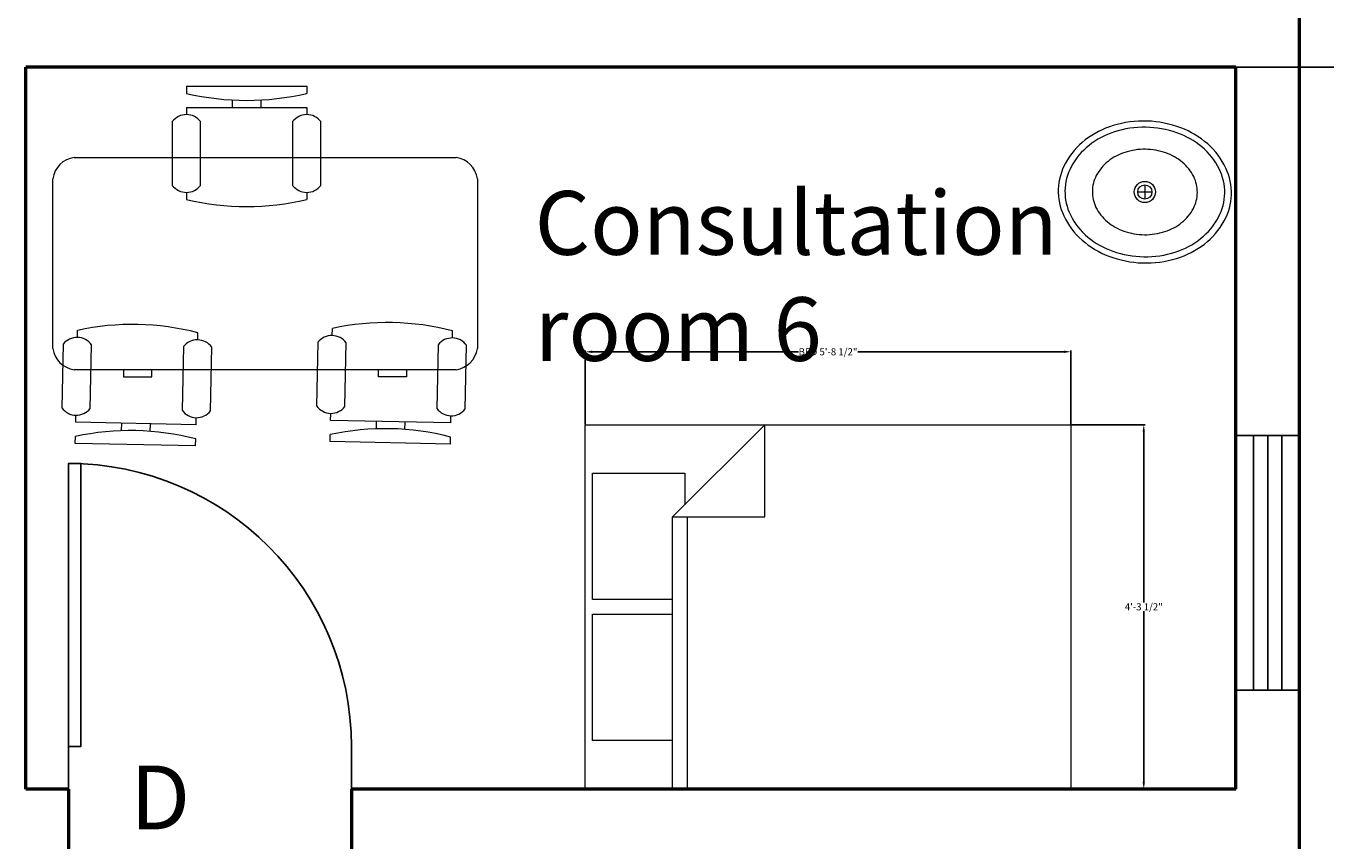
# Model space of a CAD drawing. Units: inches. Extents: x -364 to 705, y -52 to 1250.
# Tile 18 of 34: x 368 to 551, y 533 to 648. Entities that reach past the tile are written whole.
import ezdxf

# ---------------------------------------------------------------- set-up
doc = ezdxf.new("R2010")
doc.units = ezdxf.units.IN
doc.header["$MEASUREMENT"] = 0
for name, color, linetype, lineweight in [('A-ANNO-DIMS', 4, 'Continuous', 18), ('A-ANNO-IDEN', 1, 'Continuous', 18), ('A-AREA-IDEN', 3, 'Continuous', 18), ('A-DOOR', 1, 'Continuous', 25), ('A-FLOR-FIXT', 9, 'Continuous', 18), ('A-FURN', 8, 'Continuous', 18), ('A-GLAZ', 4, 'Continuous', 25), ('A-WALL', 41, 'Continuous', 50)]:
    doc.layers.add(name, color=color, linetype=linetype, lineweight=lineweight)
doc.styles.get("Standard").update_dxf_attribs({"font": 'arial.ttf'})
doc.dimstyles.get("Standard").update_dxf_attribs({"dimtxt": 1, "dimasz": 1, "dimexe": 0.18, "dimexo": 0.0625, "dimgap": 0.09, "dimtad": 0, "dimtih": 1, "dimtoh": 1, "dimdec": 0, "dimzin": 0, "dimdsep": 46, "dimlunit": 3, "dimtxsty": 'Standard', "dimcen": 0.09, "dimadec": 0, "dimazin": 0, "dimtfac": 1, "dimtdec": 0, "dimtofl": 0, "dimtmove": 0, "dimatfit": 3, "dimfxl": 1, "dimtolj": 1, "dimtzin": 0, "dimarcsym": 0})

# ---------------------------------------------------------------- blocks, each defined once
blk = doc.blocks.new('Chair - Desk')
for p, q in [((-8.5, 0), (-8.5, -1)), ((-8.5, 0), (8.5, 0)), ((8.5, 0), (8.5, -1)), ((-8.5, -3), (-8.5, -4)), ((-8.5, -3), (8.5, -3)), ((-2, -3), (-2, -1.9355)), ((2, -1.9576), (2, -3)), ((8.5, -3), (8.5, -4)), ((-10.5, -5), (-10.5, -14)), ((-6.5, -14), (-6.5, -5)), ((6.5, -5), (6.5, -14)), ((10.5, -14), (10.5, -5)), ((-8.5, -15), (-8.5, -16)), ((8.5, -15), (8.5, -16))]:
    blk.add_line(p, q)
for centre, radius, start, end in [((0, 34.625), 36.625, 256.5803, 283.4197), ((-8.5, -6.5), 2.5, 36.8699, 143.1301), ((8.5, -6.5), 2.5, 36.8699, 143.1301), ((-8.5, -12.5), 2.5, 216.8699, 323.1301), ((8.5, -12.5), 2.5, 216.8699, 323.1301), ((0, 19.625), 36.625, 256.5803, 283.4197)]:
    blk.add_arc(centre, radius, start, end)
blk = doc.blocks.new('Desk - 30 x 60 in.')
for p, q in [((-26.999995, 0), (26.999995, 0)), ((-29.999995, -27), (-29.999995, -3)), ((29.999995, -3), (29.999995, -27)), ((26.999995, -30), (-26.999995, -30)), ((-20.000005, -30), (-20.000005, -31)), ((-20.000005, -31), (-16.000005, -31)), ((-16.000005, -31), (-16.000005, -30)), ((15.999995, -31), (15.999995, -30)), ((19.999995, -31), (15.999995, -31)), ((19.999995, -30), (19.999995, -31))]:
    blk.add_line(p, q)
for centre, start, end in [((-26.499995, -3.5), 98.1301, 171.8699), ((26.499995, -3.5), 8.130102, 81.8699), ((-26.499995, -26.5), 188.1301, 261.8699), ((26.499995, -26.5), 278.1301, 351.8699)]:
    blk.add_arc(centre, 3.535534, start, end)
blk = doc.blocks.new('Bed - Queen')
for p, q in [((0, -80.00003), (0, 0)), ((0, 0), (59.99999, 0)), ((59.99999, 0), (59.99999, -80.00003)), ((7.99999, -1.2), (28.79998, -1.2)), ((7.99999, -14.4), (7.99999, -1.2)), ((28.79998, -1.2), (28.79998, -14.4)), ((31.19999, -1.2), (51.99999, -1.2)), ((31.19999, -14.4), (31.19999, -1.2)), ((51.99999, -1.2), (51.99999, -16.4)), ((0, -14.4), (44.8, -14.4)), ((59.99999, -29.6), (44.8, -14.4)), ((44.8, -14.4), (44.8, -29.6)), ((44.8, -16.8), (0, -16.8)), ((51.99999, -16.4), (46.79936, -16.4)), ((44.8, -29.6), (59.99999, -29.6)), ((59.99999, -80.00003), (0, -80.00003))]:
    blk.add_line(p, q)
blk = doc.blocks.new('*U11')
for p, q in [((0, 0), (0, -6)), ((40, 0), (40, -6))]:
    blk.add_line(p, q)
blk.add_lwpolyline([(0, 0), (0, 40), (1.75, 40), (1.75, 0)], close=True)
blk.add_arc((0, 0), 40, 0, 90)
blk = doc.blocks.new('Sink - Oval top')
for p, q in [((-1, 0), (1, 0)), ((0, 1), (0, -1))]:
    blk.add_line(p, q)
for points in [[(-12.23, 0.39, 0.117634), (-11.46, -3.36, 0.104469), (-8.88, -6.8, 0.090016), (-5.08, -9.07, 0.08192), (-0.32, -10.02, 0.08192), (4.49, -9.38, 0.090016), (8.42, -7.36, 0.104469), (11.22, -4.09, 0.117634), (12.23, -0.39, 0.117634), (11.46, 3.36, 0.104469), (8.88, 6.8, 0.090016), (5.08, 9.07, 0.08192), (0.32, 10.02, 0.08192), (-4.49, 9.38, 0.090016), (-8.42, 7.36, 0.104469), (-11.22, 4.09, 0.117634)], [(-11.29, 0.16, 0.118622), (-10.52, -3.25, 0.104678), (-8.07, -6.36, 0.089562), (-4.54, -8.37, 0.081185), (-0.13, -9.15, 0.081185), (4.3, -8.49, 0.089562), (7.89, -6.58, 0.104678), (10.42, -3.55, 0.118622), (11.29, -0.16, 0.118622), (10.52, 3.25, 0.104678), (8.07, 6.36, 0.089562), (4.54, 8.37, 0.081185), (0.13, 9.15, 0.081185), (-4.3, 8.49, 0.089562), (-7.89, 6.58, 0.104678), (-10.42, 3.55, 0.118622)], [(-7.42, 0.08, 0.118283), (-6.91, -2.17, 0.104607), (-5.29, -4.21, 0.089718), (-2.97, -5.53, 0.081436), (-0.07, -6.04, 0.081436), (2.84, -5.59, 0.089718), (5.2, -4.33, 0.104607), (6.86, -2.32, 0.118283), (7.42, -0.08, 0.118283), (6.91, 2.17, 0.104607), (5.29, 4.21, 0.089718), (2.97, 5.53, 0.081436), (0.07, 6.04, 0.081436), (-2.84, 5.59, 0.089718), (-5.2, 4.33, 0.104607), (-6.86, 2.32, 0.118283)]]:
    blk.add_lwpolyline(points, format="xyb", close=True)
for radius in [1.5, 1]:
    blk.add_circle((0, 0), radius)
blk = doc.blocks.new('WIN-36-TRIPLE-LINE')
for p, q in [((36, 6.5), (0, 6.5)), ((36, 4.5), (0, 4.5)), ((36, 2.5), (0, 2.5))]:
    blk.add_line(p, q)
blk.add_lwpolyline([(36, 0), (0, 0), (0, 9), (36, 9)], close=True)
blk = doc.blocks.new('*D58')
at = {"layer": 'A-ANNO-DIMS', "color": 0, "lineweight": -2, "transparency": 16777216}
for p, q in [((446.62, 591.66), (446.62, 602.08)), ((447.62, 601.9), (476.75, 601.9)), ((514.27, 601.9), (485.14, 601.9)), ((515.27, 591.66), (515.27, 602.08))]:
    blk.add_line(p, q, dxfattribs=at)
at = {"layer": 'A-ANNO-DIMS', "color": 0, "transparency": 16777216}
for points in [[(447.62, 602.07), (447.62, 601.73), (446.62, 601.9)], [(514.27, 602.07), (514.27, 601.73), (515.27, 601.9)]]:
    blk.add_solid(points, dxfattribs=at)
at = {"layer": 'Defpoints', "color": 0, "transparency": 16777216}
for p in [(446.62, 601.9), (446.62, 591.6), (515.27, 591.6)]:
    blk.add_point(p, dxfattribs=at)
at = {"layer": 'A-ANNO-DIMS', "color": 0, "transparency": 16777216, "insert": (480.94, 601.9), "char_height": 1, "attachment_point": 5}
blk.add_mtext('\\A1;BED 5\'-8 1/2"', dxfattribs=at)
blk = doc.blocks.new('*D59')
at = {"layer": 'A-ANNO-DIMS', "color": 0, "lineweight": -2, "transparency": 16777216}
for p, q in [((515.33, 591.6), (525.75, 591.6)), ((525.57, 590.6), (525.57, 566.47)), ((525.57, 541.11), (525.57, 565.25)), ((515.33, 540.11), (525.75, 540.11))]:
    blk.add_line(p, q, dxfattribs=at)
at = {"layer": 'A-ANNO-DIMS', "color": 0, "transparency": 16777216}
for points in [[(525.4, 590.6), (525.73, 590.6), (525.57, 591.6)], [(525.4, 541.11), (525.73, 541.11), (525.57, 540.11)]]:
    blk.add_solid(points, dxfattribs=at)
at = {"layer": 'Defpoints', "color": 0, "transparency": 16777216}
for p in [(515.27, 591.6), (525.57, 591.6), (515.27, 540.11)]:
    blk.add_point(p, dxfattribs=at)
at = {"layer": 'A-ANNO-DIMS', "color": 0, "transparency": 16777216, "insert": (525.57, 565.86), "char_height": 1, "attachment_point": 5}
blk.add_mtext('\\A1;4\'-3 1/2"', dxfattribs=at)
blk = doc.blocks.new('*D81')
at = {"layer": 'A-ANNO-DIMS', "color": 0, "lineweight": -2, "transparency": 16777216}
for p, q in [((538.64, 642.11), (703.01, 642.11)), ((702.83, 641.11), (702.83, 587.22)), ((702.83, 532.11), (702.83, 586.01)), ((538.64, 531.11), (703.01, 531.11))]:
    blk.add_line(p, q, dxfattribs=at)
at = {"layer": 'A-ANNO-DIMS', "color": 0, "transparency": 16777216}
for points in [[(702.66, 641.11), (703, 641.11), (702.83, 642.11)], [(702.66, 532.11), (703, 532.11), (702.83, 531.11)]]:
    blk.add_solid(points, dxfattribs=at)
at = {"layer": 'Defpoints', "color": 0, "transparency": 16777216}
for p in [(538.58, 642.11), (702.83, 642.11), (538.58, 531.11)]:
    blk.add_point(p, dxfattribs=at)
at = {"layer": 'A-ANNO-DIMS', "color": 0, "transparency": 16777216, "insert": (702.83, 586.61), "char_height": 1, "attachment_point": 5}
blk.add_mtext('\\A1;9\'-3"', dxfattribs=at)
blk = doc.blocks.new('*D82')
at = {"layer": 'A-ANNO-DIMS', "color": 0, "lineweight": -2, "transparency": 16777216}
for p, q in [((538.64, 753.11), (703.01, 753.11)), ((702.83, 752.11), (702.83, 698.22)), ((702.83, 643.11), (702.83, 697.01)), ((538.64, 642.11), (703.01, 642.11))]:
    blk.add_line(p, q, dxfattribs=at)
at = {"layer": 'A-ANNO-DIMS', "color": 0, "transparency": 16777216}
for points in [[(702.66, 752.11), (703, 752.11), (702.83, 753.11)], [(702.66, 643.11), (703, 643.11), (702.83, 642.11)]]:
    blk.add_solid(points, dxfattribs=at)
at = {"layer": 'Defpoints', "color": 0, "transparency": 16777216}
for p in [(538.58, 753.11), (702.83, 753.11), (538.58, 642.11)]:
    blk.add_point(p, dxfattribs=at)
at = {"layer": 'A-ANNO-DIMS', "color": 0, "transparency": 16777216, "insert": (702.83, 697.61), "char_height": 1, "attachment_point": 5}
blk.add_mtext('\\A1;9\'-3"', dxfattribs=at)

msp = doc.modelspace()

# ---------------------------------------------------------------- linework, layer by layer
at = {"layer": 'A-WALL'}
for p, q in [((547.58, 11.11), (547.58, 986.11)), ((538.58, 642.11), (367.58, 642.11)), ((379.58, 642.11), (367.58, 642.11)), ((367.58, 540.11), (367.58, 642.11)), ((538.58, 540.11), (538.58, 642.11)), ((373.58, 540.11), (367.58, 540.11)), ((373.58, 540.11), (373.58, 531.11)), ((538.58, 540.11), (413.58, 540.11)), ((413.58, 540.11), (413.58, 531.11))]:
    msp.add_line(p, q, dxfattribs=at)

# ---------------------------------------------------------------- block references
at = {"layer": 'A-DOOR'}
msp.add_blockref('*U11', (373.58, 546.11), dxfattribs=at)
at = {"layer": 'A-FLOR-FIXT'}
msp.add_blockref('Sink - Oval top', (525.72, 624.48), dxfattribs=at)
at = {"layer": 'A-FURN'}
for name, p in [('Chair - Desk', (398.76, 639.42)), ('Desk - 30 x 60 in.', (401.38, 629.36))]:
    msp.add_blockref(name, p, dxfattribs=at)
at = {"layer": 'A-FURN', "rotation": 178.8399543093713}
for p in [(419.06, 589.03), (383.05, 588.76)]:
    msp.add_blockref('Chair - Desk', p, dxfattribs=at)
at = {"layer": 'A-FURN', "xscale": 0.8581249737661522, "yscale": 0.8581249737661522, "zscale": 0.8581249737661522, "rotation": 90}
msp.add_blockref('Bed - Queen', (446.62, 540.11), dxfattribs=at)
at = {"layer": 'A-GLAZ', "rotation": 89.99999999999976}
msp.add_blockref('WIN-36-TRIPLE-LINE', (547.58, 554.08), dxfattribs=at)

# ---------------------------------------------------------------- texts
at = {"layer": 'A-ANNO-IDEN', "insert": (382.33, 543.42), "char_height": 9, "attachment_point": 1}
msp.add_mtext_dynamic_manual_height_columns('D', width=16.916, gutter_width=1, heights=[0], dxfattribs=at)
at = {"layer": 'A-AREA-IDEN', "insert": (439.48, 624.61), "char_height": 9, "attachment_point": 1}
msp.add_mtext_dynamic_manual_height_columns('Consultation room 6', width=71.704, gutter_width=1, heights=[0], dxfattribs=at)

# ---------------------------------------------------------------- dimensions: what is measured, and where the dimension line sits
at = {"layer": 'A-ANNO-DIMS'}
for base, p1, p2, picture, middle in [((702.83, 753.11), (538.58, 642.11), (538.58, 753.11), '*D82', (702.83, 697.61)), ((702.83, 642.11), (538.58, 531.11), (538.58, 642.11), '*D81', (702.83, 586.61)), ((525.57, 591.6), (515.27, 540.11), (515.27, 591.6), '*D59', (525.57, 565.86))]:
    dim = msp.add_linear_dim(base=base, p1=p1, p2=p2, angle=90, dimstyle='Standard', override={"dimdec": 1, "dimlfac": 1, "dimrnd": 0, "dimzin": 1, "dimdsep": 46, "dimlunit": 4, "dimfrac": 2}, dxfattribs=at)
    dim.commit()
    dim.dimension.update_dxf_attribs({"geometry": picture, "text_midpoint": middle})
dim = msp.add_linear_dim(base=(446.61897, 601.89965), p1=(515.269, 591.60215), p2=(446.61897, 591.60215), angle=180, text='BED <>', dimstyle='Standard', override={"dimdec": 1, "dimlfac": 1, "dimrnd": 0, "dimzin": 1, "dimdsep": 46, "dimlunit": 4, "dimfrac": 2}, dxfattribs=at)
dim.commit()
dim.dimension.update_dxf_attribs({"geometry": '*D58', "text_midpoint": (480.94399, 601.89965)})

doc.saveas('drawing.dxf')
